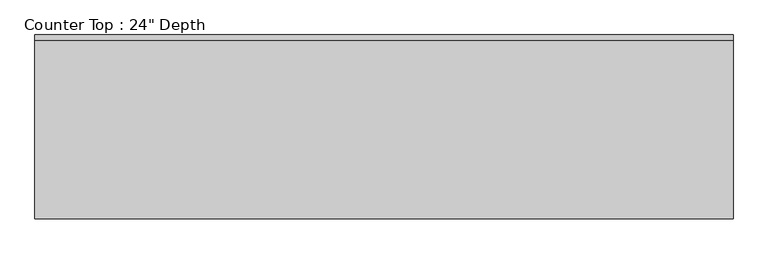
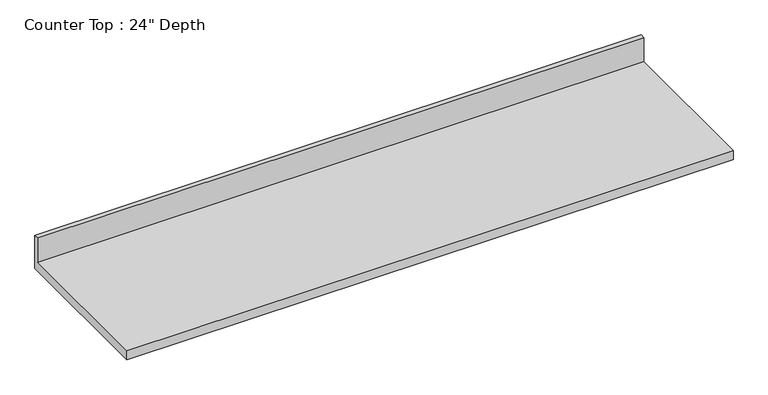
"""IFC4 building model written with IfcOpenShell, lengths in millimetres: furniture geometry."""

from ifc_helpers import new_model, si_unit, frame, origin, place, context, project, spatial, polyline, outline, extrude, source, transform, mapped, element, save


def furniture_05b7e736(model_context):
    return source(origin(), model_context, "Body", "SweptSolid", [
        extrude(outline(polyline([(0.0, 1016.0), (0.0, 876.3), (-635.0, 876.3), (-635.0, 914.4), (-19.05, 914.4), (-19.05, 1016.0), (0.0, 1016.0)])), frame((-1200.4622951, 0.0, 0.0), z_axis=(1.0, 0.0, 0.0), x_axis=(0.0, 1.0, 0.0)), (0.0, 0.0, 1.0), 2413.0),
    ])


if __name__ == "__main__":
    model = new_model("IFC4")
    model_context = context("Model", 3, world=origin())
    ifc_project = project(units=[si_unit("LENGTHUNIT", "METRE", prefix="MILLI")], contexts=[model_context])
    site = spatial("IfcSite", under=ifc_project)
    building = spatial("IfcBuilding", under=site)
    placement = place(None, origin())
    furniture_shape = furniture_05b7e736(model_context)
    element("IfcFurniture", 1, ObjectType="Counter Top : 24\" Depth", at=placement, inside=building, context=model_context, shape_type="MappedRepresentation", body=[
        mapped(furniture_shape, transform((0.0, 0.0, 0.0), x_axis=(1.0, 0.0, 0.0), y_axis=(0.0, 1.0, 0.0), z_axis=(0.0, 0.0, 1.0))),
    ])
    save(model, "model.ifc")

# Revit data of these elements
# Type "Counter Top : 24\" Depth"
#   Assembly Code = "C1030400"
#   Counter Thickness = 0' - 1 1/2"
#   Depth = 2' - 1"
#   Height = 3' - 0"
#   Length [instance default] = 8' - 0"
#   Counter Top Material = none
#   Default Elevation = 0
# Element 1 (IfcFurniture, "Counter Top : 24\" Depth")
#   Length = 7' - 11"
#   Materials on its faces: "Counter Top"
# Materials
#   "Counter Top": class "Wood", colour RGB 226 177 128, transparency 0
